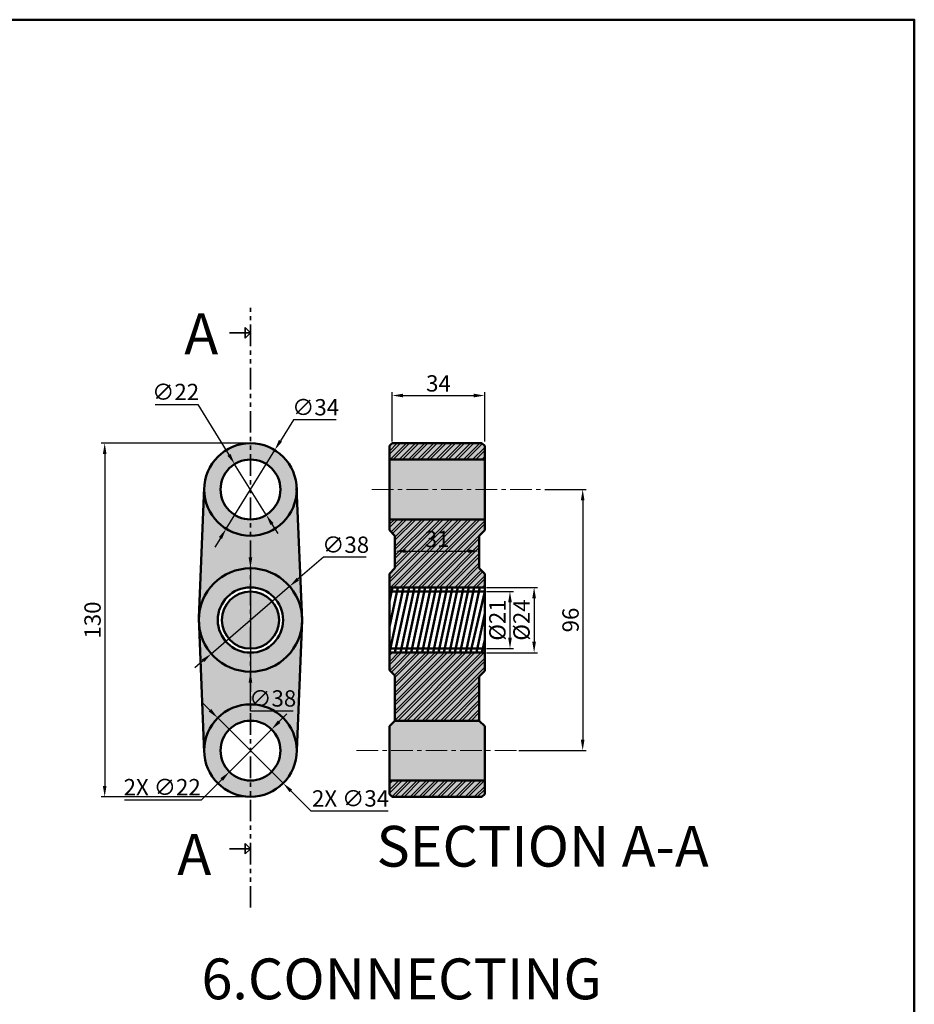
# Model space of a CAD drawing. Units: millimetres. Extents: x -14 to 1073, y -445 to 318.
# Tile 6 of 6: x 744 to 1073, y -44 to 318. Entities that reach past the tile are written whole.
import ezdxf

# ---------------------------------------------------------------- set-up
doc = ezdxf.new("R2010")
doc.units = ezdxf.units.MM
doc.header["$LTSCALE"] = 0.5
doc.linetypes.add('CENTER', pattern=[50.8, 31.75, -6.35, 6.35, -6.35])
doc.linetypes.add('PHANTOM', pattern=[63.5, 31.75, -6.35, 6.35, -6.35, 6.35, -6.35])
for name, color, linetype, lineweight in [('M-CNTR', 1, 'CENTER', 18), ('M-DIMS', 2, 'Continuous', 25), ('M-HATC', 8, 'Continuous', 18), ('M-OUTL', 7, 'Continuous', 50), ('M-SECT', 6, 'PHANTOM', 35), ('M-TEXT', 3, 'Continuous', 25)]:
    doc.layers.add(name, color=color, linetype=linetype, lineweight=lineweight)
doc.styles.get("Standard").update_dxf_attribs({"font": 'arial.ttf'})
doc.dimstyles.new('ISO-25', dxfattribs={"dimtxt": 6, "dimasz": 4, "dimexe": 1.25, "dimexo": 0.625, "dimtad": 1, "dimtoh": 1, "dimtxsty": 'Standard', "dimcen": 2.5, "dimadec": 0, "dimazin": 0, "dimtfac": 1, "dimtmove": 0, "dimatfit": 3, "dimfxl": 1, "dimarcsym": 0})
pattern_1 = [(45, (-73.225, 317.7532), (-1.683798, 1.683798), []), (45, (-72.1024, 317.7532), (-1.683798, 1.683798), [])]

# ---------------------------------------------------------------- blocks, each defined once
blk = doc.blocks.new('*D62')
at = {"layer": 'Defpoints', "color": 0, "ltscale": 0.5, "transparency": 16777216}
for p in [(914.86, 179.93), (880.86, 162.41), (914.86, 162.41)]:
    blk.add_point(p, dxfattribs=at)
at = {"layer": 'M-DIMS', "color": 0, "lineweight": -2, "ltscale": 0.5, "transparency": 16777216}
for p, q in [((880.86, 163.04), (880.86, 181.18)), ((914.86, 163.04), (914.86, 181.18)), ((884.86, 179.93), (910.86, 179.93))]:
    blk.add_line(p, q, dxfattribs=at)
at = {"layer": 'M-DIMS', "color": 0, "ltscale": 0.5, "transparency": 16777216}
for points in [[(884.86, 180.6), (884.86, 179.27), (880.86, 179.93)], [(910.86, 180.6), (910.86, 179.27), (914.86, 179.93)]]:
    blk.add_solid(points, dxfattribs=at)
at = {"layer": 'M-DIMS', "color": 0, "ltscale": 0.5, "transparency": 16777216, "insert": (897.86, 183.62), "char_height": 6, "attachment_point": 5}
blk.add_mtext('34', dxfattribs=at)
blk = doc.blocks.new('*D63')
at = {"layer": 'Defpoints', "color": 0, "ltscale": 0.5, "transparency": 16777216}
for p in [(914.86, 109.41), (914.86, 85.41), (933.02, 85.41)]:
    blk.add_point(p, dxfattribs=at)
at = {"layer": 'M-DIMS', "color": 0, "lineweight": -2, "ltscale": 0.5, "transparency": 16777216}
for p, q in [((915.49, 109.41), (934.27, 109.41)), ((933.02, 105.41), (933.02, 89.41)), ((915.49, 85.41), (934.27, 85.41))]:
    blk.add_line(p, q, dxfattribs=at)
at = {"layer": 'M-DIMS', "color": 0, "ltscale": 0.5, "transparency": 16777216}
for points in [[(932.35, 105.41), (933.68, 105.41), (933.02, 109.41)], [(932.35, 89.41), (933.68, 89.41), (933.02, 85.41)]]:
    blk.add_solid(points, dxfattribs=at)
at = {"layer": 'M-DIMS', "color": 0, "ltscale": 0.5, "transparency": 16777216, "insert": (929.16, 97.41), "char_height": 6, "attachment_point": 5, "rotation": 90}
blk.add_mtext('%%C24', dxfattribs=at)
blk = doc.blocks.new('*D64')
at = {"layer": 'Defpoints', "color": 0, "ltscale": 0.5, "transparency": 16777216}
for p in [(914.86, 107.91), (914.86, 86.91), (924.15, 86.91)]:
    blk.add_point(p, dxfattribs=at)
at = {"layer": 'M-DIMS', "color": 0, "lineweight": -2, "ltscale": 0.5, "transparency": 16777216}
for p, q in [((915.49, 107.91), (925.4, 107.91)), ((924.15, 103.91), (924.15, 90.91)), ((915.49, 86.91), (925.4, 86.91))]:
    blk.add_line(p, q, dxfattribs=at)
at = {"layer": 'M-DIMS', "color": 0, "ltscale": 0.5, "transparency": 16777216}
for points in [[(923.48, 103.91), (924.82, 103.91), (924.15, 107.91)], [(923.48, 90.91), (924.82, 90.91), (924.15, 86.91)]]:
    blk.add_solid(points, dxfattribs=at)
at = {"layer": 'M-DIMS', "color": 0, "ltscale": 0.5, "transparency": 16777216, "insert": (920.29, 97.41), "char_height": 6, "attachment_point": 5, "rotation": 90}
blk.add_mtext('%%C21', dxfattribs=at)
blk = doc.blocks.new('*D65')
at = {"layer": 'Defpoints', "color": 0, "ltscale": 0.5, "transparency": 16777216}
for p in [(837.69, 159.88), (819.83, 130.94)]:
    blk.add_point(p, dxfattribs=at)
at = {"layer": 'M-DIMS', "color": 0, "lineweight": -2, "ltscale": 0.5, "transparency": 16777216}
for p, q in [((844.55, 171), (839.79, 163.28)), ((860.27, 171), (844.55, 171)), ((819.83, 130.94), (837.69, 159.88)), ((817.73, 127.54), (815.63, 124.14))]:
    blk.add_line(p, q, dxfattribs=at)
at = {"layer": 'M-DIMS', "color": 0, "ltscale": 0.5, "transparency": 16777216}
for points in [[(839.22, 163.63), (840.36, 162.93), (837.69, 159.88)], [(817.16, 127.89), (818.3, 127.19), (819.83, 130.94)]]:
    blk.add_solid(points, dxfattribs=at)
at = {"layer": 'M-DIMS', "color": 0, "ltscale": 0.5, "transparency": 16777216, "insert": (852.72, 174.85), "char_height": 6, "attachment_point": 5}
blk.add_mtext('∅34', dxfattribs=at)
blk = doc.blocks.new('*D66')
at = {"layer": 'Defpoints', "color": 0, "ltscale": 0.5, "transparency": 16777216}
for p in [(822.96, 154.76), (834.56, 136.06)]:
    blk.add_point(p, dxfattribs=at)
at = {"layer": 'M-DIMS', "color": 0, "lineweight": -2, "ltscale": 0.5, "transparency": 16777216}
for p, q in [((793.73, 176.62), (809.41, 176.62)), ((809.41, 176.62), (820.86, 158.16)), ((834.56, 136.06), (822.96, 154.76)), ((836.66, 132.66), (838.77, 129.26))]:
    blk.add_line(p, q, dxfattribs=at)
at = {"layer": 'M-DIMS', "color": 0, "ltscale": 0.5, "transparency": 16777216}
for points in [[(821.42, 158.51), (820.29, 157.81), (822.96, 154.76)], [(837.23, 133.01), (836.1, 132.31), (834.56, 136.06)]]:
    blk.add_solid(points, dxfattribs=at)
at = {"layer": 'M-DIMS', "color": 0, "ltscale": 0.5, "transparency": 16777216, "insert": (801.26, 180.47), "char_height": 6, "attachment_point": 5}
blk.add_mtext('∅22', dxfattribs=at)
blk = doc.blocks.new('*D67')
at = {"layer": 'Defpoints', "color": 0, "ltscale": 0.5, "transparency": 16777216}
for p in [(843.16, 109.8), (814.36, 85.02)]:
    blk.add_point(p, dxfattribs=at)
at = {"layer": 'M-DIMS', "color": 0, "lineweight": -2, "ltscale": 0.5, "transparency": 16777216}
for p, q in [((855.55, 120.46), (846.2, 112.41)), ((871.31, 120.46), (855.55, 120.46)), ((814.36, 85.02), (843.16, 109.8)), ((811.32, 82.41), (808.29, 79.8))]:
    blk.add_line(p, q, dxfattribs=at)
at = {"layer": 'M-DIMS', "color": 0, "ltscale": 0.5, "transparency": 16777216}
for points in [[(845.76, 112.92), (846.63, 111.91), (843.16, 109.8)], [(810.89, 82.92), (811.76, 81.91), (814.36, 85.02)]]:
    blk.add_solid(points, dxfattribs=at)
at = {"layer": 'M-DIMS', "color": 0, "ltscale": 0.5, "transparency": 16777216, "insert": (863.75, 124.32), "char_height": 6, "attachment_point": 5}
blk.add_mtext('∅38', dxfattribs=at)
blk = doc.blocks.new('*D68')
at = {"layer": 'Defpoints', "color": 0, "ltscale": 0.5, "transparency": 16777216}
for p in [(828.76, 162.41), (775.19, 32.41), (828.76, 32.41)]:
    blk.add_point(p, dxfattribs=at)
at = {"layer": 'M-DIMS', "color": 0, "lineweight": -2, "ltscale": 0.5, "transparency": 16777216}
for p, q in [((828.13, 162.41), (773.94, 162.41)), ((775.19, 158.41), (775.19, 36.41)), ((828.13, 32.41), (773.94, 32.41))]:
    blk.add_line(p, q, dxfattribs=at)
at = {"layer": 'M-DIMS', "color": 0, "ltscale": 0.5, "transparency": 16777216}
for points in [[(774.53, 158.41), (775.86, 158.41), (775.19, 162.41)], [(774.53, 36.41), (775.86, 36.41), (775.19, 32.41)]]:
    blk.add_solid(points, dxfattribs=at)
at = {"layer": 'M-DIMS', "color": 0, "ltscale": 0.5, "transparency": 16777216, "insert": (771.5, 97.41), "char_height": 6, "attachment_point": 5, "rotation": 90}
blk.add_mtext('130', dxfattribs=at)
blk = doc.blocks.new('*D69')
at = {"layer": 'Defpoints', "color": 0, "ltscale": 0.5, "transparency": 16777216}
for p in [(881.86, 122.41), (912.86, 122.73), (912.86, 122.41)]:
    blk.add_point(p, dxfattribs=at)
at = {"layer": 'M-DIMS', "color": 0, "lineweight": -2, "ltscale": 0.5, "transparency": 16777216}
for p, q in [((881.86, 123.04), (881.86, 123.98)), ((912.86, 123.04), (912.86, 123.98)), ((885.86, 122.73), (908.86, 122.73))]:
    blk.add_line(p, q, dxfattribs=at)
at = {"layer": 'M-DIMS', "color": 0, "ltscale": 0.5, "transparency": 16777216}
for points in [[(885.86, 123.39), (885.86, 122.06), (881.86, 122.73)], [(908.86, 123.39), (908.86, 122.06), (912.86, 122.73)]]:
    blk.add_solid(points, dxfattribs=at)
at = {"layer": 'M-DIMS', "color": 0, "ltscale": 0.5, "transparency": 16777216, "insert": (897.36, 126.42), "char_height": 6, "attachment_point": 5}
blk.add_mtext('31', dxfattribs=at)
blk = doc.blocks.new('*D79')
at = {"layer": 'Defpoints', "color": 0, "ltscale": 0.5, "transparency": 16777216}
for p in [(936.27, 145.41), (926.82, 49.41), (950.87, 49.41)]:
    blk.add_point(p, dxfattribs=at)
at = {"layer": 'M-DIMS', "color": 0, "lineweight": -2, "ltscale": 0.5, "transparency": 16777216}
for p, q in [((936.9, 145.41), (952.12, 145.41)), ((950.87, 141.41), (950.87, 53.41)), ((927.44, 49.41), (952.12, 49.41))]:
    blk.add_line(p, q, dxfattribs=at)
at = {"layer": 'M-DIMS', "color": 0, "ltscale": 0.5, "transparency": 16777216}
for points in [[(950.2, 141.41), (951.54, 141.41), (950.87, 145.41)], [(950.2, 53.41), (951.54, 53.41), (950.87, 49.41)]]:
    blk.add_solid(points, dxfattribs=at)
at = {"layer": 'M-DIMS', "color": 0, "ltscale": 0.5, "transparency": 16777216, "insert": (947.18, 97.41), "char_height": 6, "attachment_point": 5, "rotation": 90}
blk.add_mtext('96', dxfattribs=at)
blk = doc.blocks.new('*D91')
at = {"layer": 'Defpoints', "color": 0, "ltscale": 0.5, "transparency": 16777216}
for p in [(836.51, 57.22), (821.01, 41.61)]:
    blk.add_point(p, dxfattribs=at)
at = {"layer": 'M-DIMS', "color": 0, "lineweight": -2, "ltscale": 0.5, "transparency": 16777216}
for p, q in [((839.33, 60.05), (842.15, 62.89)), ((836.51, 57.22), (821.01, 41.61)), ((810.82, 31.35), (818.19, 38.77)), ((782.45, 31.35), (810.82, 31.35))]:
    blk.add_line(p, q, dxfattribs=at)
at = {"layer": 'M-DIMS', "color": 0, "ltscale": 0.5, "transparency": 16777216}
for points in [[(838.86, 60.52), (839.8, 59.58), (836.51, 57.22)], [(817.72, 39.24), (818.66, 38.3), (821.01, 41.61)]]:
    blk.add_solid(points, dxfattribs=at)
at = {"layer": 'M-DIMS', "color": 0, "ltscale": 0.5, "transparency": 16777216, "insert": (796.32, 35.2), "char_height": 6, "attachment_point": 5}
blk.add_mtext('2X ∅22', dxfattribs=at)
blk = doc.blocks.new('*D92')
at = {"layer": 'Defpoints', "color": 0, "ltscale": 0.5, "transparency": 16777216}
for p in [(816.72, 61.42), (840.79, 37.41)]:
    blk.add_point(p, dxfattribs=at)
at = {"layer": 'M-DIMS', "color": 0, "lineweight": -2, "ltscale": 0.5, "transparency": 16777216}
for p, q in [((813.89, 64.24), (811.06, 67.07)), ((816.72, 61.42), (840.79, 37.41)), ((851.03, 27.19), (843.63, 34.58)), ((879.43, 27.19), (851.03, 27.19))]:
    blk.add_line(p, q, dxfattribs=at)
at = {"layer": 'M-DIMS', "color": 0, "ltscale": 0.5, "transparency": 16777216}
for points in [[(814.36, 64.71), (813.42, 63.77), (816.72, 61.42)], [(844.1, 35.05), (843.16, 34.11), (840.79, 37.41)]]:
    blk.add_solid(points, dxfattribs=at)
at = {"layer": 'M-DIMS', "color": 0, "ltscale": 0.5, "transparency": 16777216, "insert": (865.55, 31.05), "char_height": 6, "attachment_point": 5}
blk.add_mtext('2X ∅34', dxfattribs=at)
blk = doc.blocks.new('*D93')
at = {"layer": 'Defpoints', "color": 0, "ltscale": 0.5, "transparency": 16777216}
for p in [(828.76, 116.41), (828.76, 78.41)]:
    blk.add_point(p, dxfattribs=at)
at = {"layer": 'M-DIMS', "color": 0, "lineweight": -2, "ltscale": 0.5, "transparency": 16777216}
for p, q in [((828.76, 120.41), (828.76, 124.41)), ((828.76, 116.41), (828.76, 78.41)), ((828.76, 63.95), (828.76, 74.41)), ((844.52, 63.95), (828.76, 63.95))]:
    blk.add_line(p, q, dxfattribs=at)
at = {"layer": 'M-DIMS', "color": 0, "ltscale": 0.5, "transparency": 16777216}
for points in [[(829.42, 120.41), (828.09, 120.41), (828.76, 116.41)], [(829.43, 74.41), (828.09, 74.41), (828.76, 78.41)]]:
    blk.add_solid(points, dxfattribs=at)
at = {"layer": 'M-DIMS', "color": 0, "ltscale": 0.5, "transparency": 16777216, "insert": (836.95, 67.81), "char_height": 6, "attachment_point": 5}
blk.add_mtext('∅38', dxfattribs=at)

msp = doc.modelspace()

# ---------------------------------------------------------------- hatches: boundary and pattern name
at = {"layer": 'M-HATC', "ltscale": 0.5}
h = msp.add_hatch(color=256, dxfattribs=at)
h.set_gradient(color1=(69, 84, 165), color2=(69, 84, 165), name='INVCYLINDER')
h.paths.add_polyline_path([(847.6934, 95.831, -0.90211761), (809.9013, 95.0923), (811.7731, 48.7259, -0.01008703), (811.7592, 49.4116, -1), (845.7592, 49.4116)])
h.paths.add_polyline_path([(845.7592, 49.4116, 1), (811.7592, 49.4116, 1)])
h.paths.add_polyline_path([(817.7592, 49.4116, -1), (839.7592, 49.4116, -1)], flags=16)
h.paths.add_polyline_path([(847.6934, 95.831), (847.7592, 97.4116), (847.6943, 98.9807, 0.9396764), (809.7757, 98.2033), (809.9013, 95.0923, 0.90211761)])
h.paths.add_polyline_path([(816.7592, 97.4116, -1), (840.7592, 97.4116, -1)], flags=16)
h.paths.add_polyline_path([(818.2592, 97.4116, -1), (839.2592, 97.4116, -1)], flags=0)
h.paths.add_polyline_path([(845.7447, 146.1142, -0.01033543), (845.7592, 145.4116, -1), (811.7592, 145.4116, -0.01042006), (811.774, 146.1199), (809.7757, 98.2033, -0.9396764), (847.6943, 98.9807)])
h.paths.add_polyline_path([(811.7592, 145.4116, 1), (845.7592, 145.4116, 1)])
h.paths.add_polyline_path([(839.7592, 145.4116, -1), (817.7592, 145.4116, -1)], flags=16)
h = msp.add_hatch(dxfattribs=at)
h.set_pattern_fill('ANSI32', color=256, scale=0.25, style=0)
h.set_pattern_definition(pattern_1)
h.paths.add_polyline_path([(914.8628, 156.4116), (914.8628, 161.4116), (913.8628, 162.4116), (880.8628, 162.4116), (879.8628, 161.4116), (879.8628, 156.4116)])
h.paths.add_polyline_path([(879.8628, 134.4116), (879.8628, 130.4116), (881.8628, 128.4116), (881.8628, 116.4116), (879.8628, 114.4116), (879.8628, 109.4116), (914.8628, 109.4116), (914.8628, 114.4116), (912.8628, 116.4116), (912.8628, 128.4116), (914.8628, 130.4116), (914.8628, 134.4116)])
h.paths.add_polyline_path([(912.8628, 60.4116), (912.8628, 76.6795), (914.8628, 78.6795), (914.8628, 85.4116), (879.8628, 85.4116), (879.8628, 78.9857), (881.8628, 76.9857), (881.8628, 60.4116)])
h.paths.add_polyline_path([(913.8628, 32.4116), (914.8628, 33.4116), (914.8628, 38.4116), (879.8628, 38.4116), (879.8628, 33.4116), (880.8628, 32.4116)])
h = msp.add_hatch(color=256, dxfattribs=at)
h.set_gradient(color1=(41, 49, 137), color2=(41, 49, 137), name='INVCYLINDER')
h.paths.add_polyline_path([(914.8628, 156.4116), (879.8628, 156.4116), (879.8628, 145.4116), (914.8628, 145.4116)])
h.paths.add_polyline_path([(914.8628, 145.4116), (879.8628, 145.4116), (879.8628, 134.4116), (914.8628, 134.4116)])
h.paths.add_polyline_path([(914.8628, 58.4116), (912.8628, 60.4116), (881.8628, 60.4116), (879.8628, 58.4116), (879.8628, 49.4116), (914.8628, 49.4116)])
h.paths.add_polyline_path([(914.8628, 49.4116), (879.8628, 49.4116), (879.8628, 38.4116), (914.8628, 38.4116)])
h.paths.add_polyline_path([(914.8628, 130.4116), (914.8628, 134.4116), (879.8628, 134.4116), (879.8628, 130.4116), (881.8628, 128.4116), (881.8628, 116.4116), (879.8628, 114.4116), (879.8628, 109.4116), (914.8628, 109.4116), (914.8628, 114.4116), (912.8628, 116.4116), (912.8628, 128.4116)])
h.paths.add_polyline_path([(914.8628, 161.4116), (913.8628, 162.4116), (880.8628, 162.4116), (879.8628, 161.4116), (879.8628, 156.4116), (914.8628, 156.4116)])
h.paths.add_polyline_path([(912.8628, 76.6795), (914.8628, 78.6795), (914.8628, 85.4116), (879.8628, 85.4116), (879.8628, 78.9857), (881.8628, 76.9857), (881.8628, 60.4116), (912.8628, 60.4116)])
h.paths.add_polyline_path([(914.8628, 38.4116), (879.8628, 38.4116), (879.8628, 33.4116), (880.8628, 32.4116), (913.8628, 32.4116), (914.8628, 33.4116)])
h = msp.add_hatch(dxfattribs=at)
h.set_pattern_fill('ANSI32', color=256, scale=0.25, style=0)
h.set_pattern_definition(pattern_1)
h.paths.add_polyline_path([(879.8628, 156.4116), (914.8628, 156.4116), (914.8628, 161.4116), (913.8628, 162.4116), (880.8628, 162.4116), (879.8628, 161.4116)])
h.paths.add_polyline_path([(914.8628, 130.4116), (914.8628, 134.4116), (879.8628, 134.4116), (879.8628, 130.4116), (881.8628, 128.4116), (881.8628, 116.4116), (879.8628, 114.4116), (879.8628, 109.4116), (914.8628, 109.4116), (914.8628, 114.4116), (912.8628, 116.4116), (912.8628, 128.4116)])
h.paths.add_polyline_path([(879.8628, 85.4116), (879.8628, 78.9857), (881.8628, 76.9857), (881.8628, 60.4116), (912.8628, 60.4116), (912.8628, 76.6795), (914.8628, 78.6795), (914.8628, 85.4116)])
h.paths.add_polyline_path([(914.8628, 33.4116), (914.8628, 38.4116), (879.8628, 38.4116), (879.8628, 33.4116), (880.8628, 32.4116), (913.8628, 32.4116)])

# ---------------------------------------------------------------- linework, layer by layer
at = {"layer": 'M-CNTR', "ltscale": 0.5}
for p, q in [((873.4092, 145.4116), (936.2701, 145.4116)), ((867.769, 49.4116), (926.8176, 49.4116))]:
    msp.add_line(p, q, dxfattribs=at)
at = {"layer": 'M-OUTL', "ltscale": 0.5}
for p, q in [((880.8628, 162.4116), (879.8628, 161.4116)), ((879.8628, 161.4116), (879.8628, 130.4116)), ((913.8628, 162.4116), (880.8628, 162.4116)), ((913.8628, 162.4116), (914.8628, 161.4116)), ((914.8628, 130.4116), (914.8628, 161.4116)), ((879.8628, 156.4116), (914.8628, 156.4116)), ((811.774, 146.1199), (809.7757, 98.2033)), ((845.7447, 146.1142), (847.7592, 97.4116)), ((879.8628, 134.4116), (914.8628, 134.4116)), ((881.8628, 128.4116), (879.8628, 130.4116)), ((912.8628, 128.4116), (914.8628, 130.4116)), ((881.8628, 128.4116), (881.8628, 116.4116)), ((912.8628, 128.4116), (912.8628, 116.4116)), ((881.8628, 116.4116), (879.8628, 114.4116)), ((912.8628, 116.4116), (914.8628, 114.4116)), ((879.8628, 114.4116), (879.8628, 78.9857)), ((914.8628, 78.6795), (914.8628, 114.4116)), ((879.8628, 109.4116), (914.8628, 109.4116)), ((885.0357, 109.4116), (879.8628, 85.4116)), ((882.9898, 109.4116), (879.8628, 94.9037)), ((880.9438, 109.4116), (879.8628, 104.3959)), ((887.0357, 109.4116), (881.8628, 85.4116)), ((889.0357, 109.4116), (883.8628, 85.4116)), ((885.0357, 109.4116), (885.0357, 109.4116)), ((891.0357, 109.4116), (885.8628, 85.4116)), ((893.0357, 109.4116), (887.8628, 85.4116)), ((895.0357, 109.4116), (889.8628, 85.4116)), ((897.0357, 109.4116), (891.8628, 85.4116)), ((899.0357, 109.4116), (893.8628, 85.4116)), ((901.0357, 109.4116), (895.8628, 85.4116)), ((903.0357, 109.4116), (897.8628, 85.4116)), ((905.0357, 109.4116), (899.8628, 85.4116)), ((907.0357, 109.4116), (901.8628, 85.4116)), ((907.0357, 109.4116), (901.8628, 85.4116)), ((909.0357, 109.4116), (903.8628, 85.4116)), ((911.0357, 109.4116), (905.8628, 85.4116)), ((913.0357, 109.4116), (907.8628, 85.4116)), ((879.8628, 107.9116), (914.8628, 107.9116)), ((914.8628, 107.9116), (909.6378, 85.4116)), ((809.7757, 98.2033), (811.7731, 48.7259)), ((914.8628, 99.8512), (911.8152, 85.4116)), ((847.7592, 97.4116), (845.7592, 49.4116)), ((879.8628, 86.9116), (914.8628, 86.9116)), ((914.8628, 90.1662), (913.8593, 85.4116)), ((879.8628, 85.4116), (914.8628, 85.4116)), ((879.8628, 78.9857), (881.8628, 76.9857)), ((881.8628, 76.9857), (881.8628, 60.4116)), ((914.8628, 78.6795), (912.8628, 76.6795)), ((912.8628, 76.6795), (912.8628, 60.4116)), ((881.8628, 60.4116), (879.8628, 58.4116)), ((879.8628, 58.4116), (879.8628, 33.4116)), ((881.8628, 60.4116), (912.8628, 60.4116)), ((912.8628, 60.4116), (914.8628, 58.4116)), ((914.8628, 33.4116), (914.8628, 58.4116)), ((879.8628, 38.4116), (914.8628, 38.4116)), ((879.8628, 33.4116), (880.8628, 32.4116)), ((913.8628, 32.4116), (914.8628, 33.4116)), ((880.8628, 32.4116), (913.8628, 32.4116))]:
    msp.add_line(p, q, dxfattribs=at)
msp.add_lwpolyline([(-13.7695, 318.0907), (1072.7514, 318.0907), (1072.7514, -445.1795), (-13.7695, -445.1795)], close=True, dxfattribs=at)
for centre, radius in [((828.7592, 145.4116), 17), ((828.7592, 145.4116), 11), ((828.7592, 97.4116), 19), ((828.7592, 97.4116), 12), ((828.7592, 97.4116), 10.5), ((828.7592, 49.4116), 17), ((828.7592, 49.4116), 11)]:
    msp.add_circle(centre, radius, dxfattribs=at)
at = {"layer": 'M-SECT', "ltscale": 0.5}
for p, q in [((828.7592, -8.3198), (828.7592, 212.1927)), ((821.0665, 202.9944), (828.7592, 202.9944)), ((826.836, 201.0712), (826.836, 204.9176)), ((828.7592, 202.9944), (826.836, 204.9176)), ((828.7592, 202.9944), (826.836, 201.0712)), ((826.836, 11.4292), (826.836, 15.2756)), ((828.7592, 13.3524), (826.836, 15.2756)), ((821.0665, 13.3524), (828.7592, 13.3524)), ((828.7592, 13.3524), (826.836, 11.4292)), ((828.7592, 13.3524), (828.7592, 13.3524))]:
    msp.add_line(p, q, dxfattribs=at)

# ---------------------------------------------------------------- texts
at = {"layer": 'M-TEXT', "ltscale": 0.5, "char_height": 15, "attachment_point": 1}
for s, width, insert in [('A', 18.40709, (804.4555, 210.1366)), ('\\pxqc;SECTION A-A', 136.631013, (867.8407, 21.7426)), ('A', 18.40709, (801.8934, 18.7425)), ('\\pxqc;6.CONNECTING WEDGE', 218.927832, (774.8768, -27.0126))]:
    msp.add_mtext_dynamic_manual_height_columns(s, width=width, gutter_width=12.5, heights=[0], dxfattribs=dict(at, insert=insert))

# ---------------------------------------------------------------- dimensions: what is measured, and where the dimension line sits
at = {"layer": 'M-DIMS', "ltscale": 0.5}
for base, p1, p2, picture, middle in [((914.8628, 179.9318), (880.8628, 162.4116), (914.8628, 162.4116), '*D62', (897.8628, 183.6223)), ((912.8628, 122.7255), (881.8628, 122.4116), (912.8628, 122.4116), '*D69', (897.3628, 126.416))]:
    dim = msp.add_linear_dim(base=base, p1=p1, p2=p2, dimstyle='ISO-25', override={"dimclrd": 0, "dimclre": 0, "dimclrt": 0}, dxfattribs=at)
    dim.commit()
    dim.dimension.update_dxf_attribs({"geometry": picture, "text_midpoint": middle})
for p1, p2, override, picture, middle in [((834.5554, 136.0626), (822.963, 154.7606), {"dimclrd": 0, "dimclre": 0, "dimclrt": 0}, '*D66', (801.258, 176.6151)), ((819.8308, 130.945), (837.6876, 159.8782), {"dimclrd": 0, "dimclre": 0, "dimclrt": 0}, '*D65', (852.7248, 170.9983)), ((814.3552, 85.0211), (843.1633, 109.802), {"dimclrd": 0, "dimclre": 0, "dimclrt": 0}, '*D67', (863.7453, 120.4596)), ((828.7584, 116.4116), (828.76, 78.4116), {"dimdec": 0, "dimlfac": 1, "dimrnd": 0, "dimzin": 0, "dimdsep": 46, "dimlunit": 2}, '*D93', (836.9531, 63.9491))]:
    dim = msp.add_diameter_dim_2p(p1=p1, p2=p2, dimstyle='ISO-25', override=override, dxfattribs=at)
    dim.commit()
    dim.dimension.update_dxf_attribs({"geometry": picture, "text_midpoint": middle, "dimtype": 163})
for base, p1, p2, override, picture, middle in [((775.1947, 32.4116), (828.7592, 162.4116), (828.7592, 32.4116), {"dimclrd": 0, "dimclre": 0, "dimclrt": 0}, '*D68', (771.5042, 97.4116)), ((950.8701, 49.4116), (936.2701, 145.4116), (926.8176, 49.4116), {"dimdec": 0, "dimlfac": 1, "dimrnd": 0, "dimzin": 0, "dimdsep": 46, "dimlunit": 2}, '*D79', (947.1817, 97.4116))]:
    dim = msp.add_linear_dim(base=base, p1=p1, p2=p2, angle=90, dimstyle='ISO-25', override=override, dxfattribs=at)
    dim.commit()
    dim.dimension.update_dxf_attribs({"geometry": picture, "text_midpoint": middle})
for base, p1, p2, picture, middle in [((933.0181, 85.4116), (914.8628, 109.4116), (914.8628, 85.4116), '*D63', (929.1618, 97.4116)), ((924.149, 86.9116), (914.8628, 107.9116), (914.8628, 86.9116), '*D64', (920.2928, 97.4116))]:
    dim = msp.add_linear_dim(base=base, p1=p1, p2=p2, angle=90, text='%%C<>', dimstyle='ISO-25', override={"dimclrd": 0, "dimclre": 0, "dimclrt": 0}, dxfattribs=at)
    dim.commit()
    dim.dimension.update_dxf_attribs({"geometry": picture, "text_midpoint": middle})
for p1, p2, picture, middle in [((816.7238, 61.4178), (840.7946, 37.4054), '*D92', (865.5453, 27.1913)), ((836.5112, 57.2159), (821.0072, 41.6073), '*D91', (796.3218, 31.3464))]:
    dim = msp.add_diameter_dim_2p(p1=p1, p2=p2, text='2X <>', dimstyle='ISO-25', override={"dimdec": 0, "dimlfac": 1, "dimrnd": 0, "dimzin": 0, "dimdsep": 46, "dimlunit": 2}, dxfattribs=at)
    dim.commit()
    dim.dimension.update_dxf_attribs({"geometry": picture, "text_midpoint": middle, "dimtype": 163})

doc.saveas('drawing.dxf')
